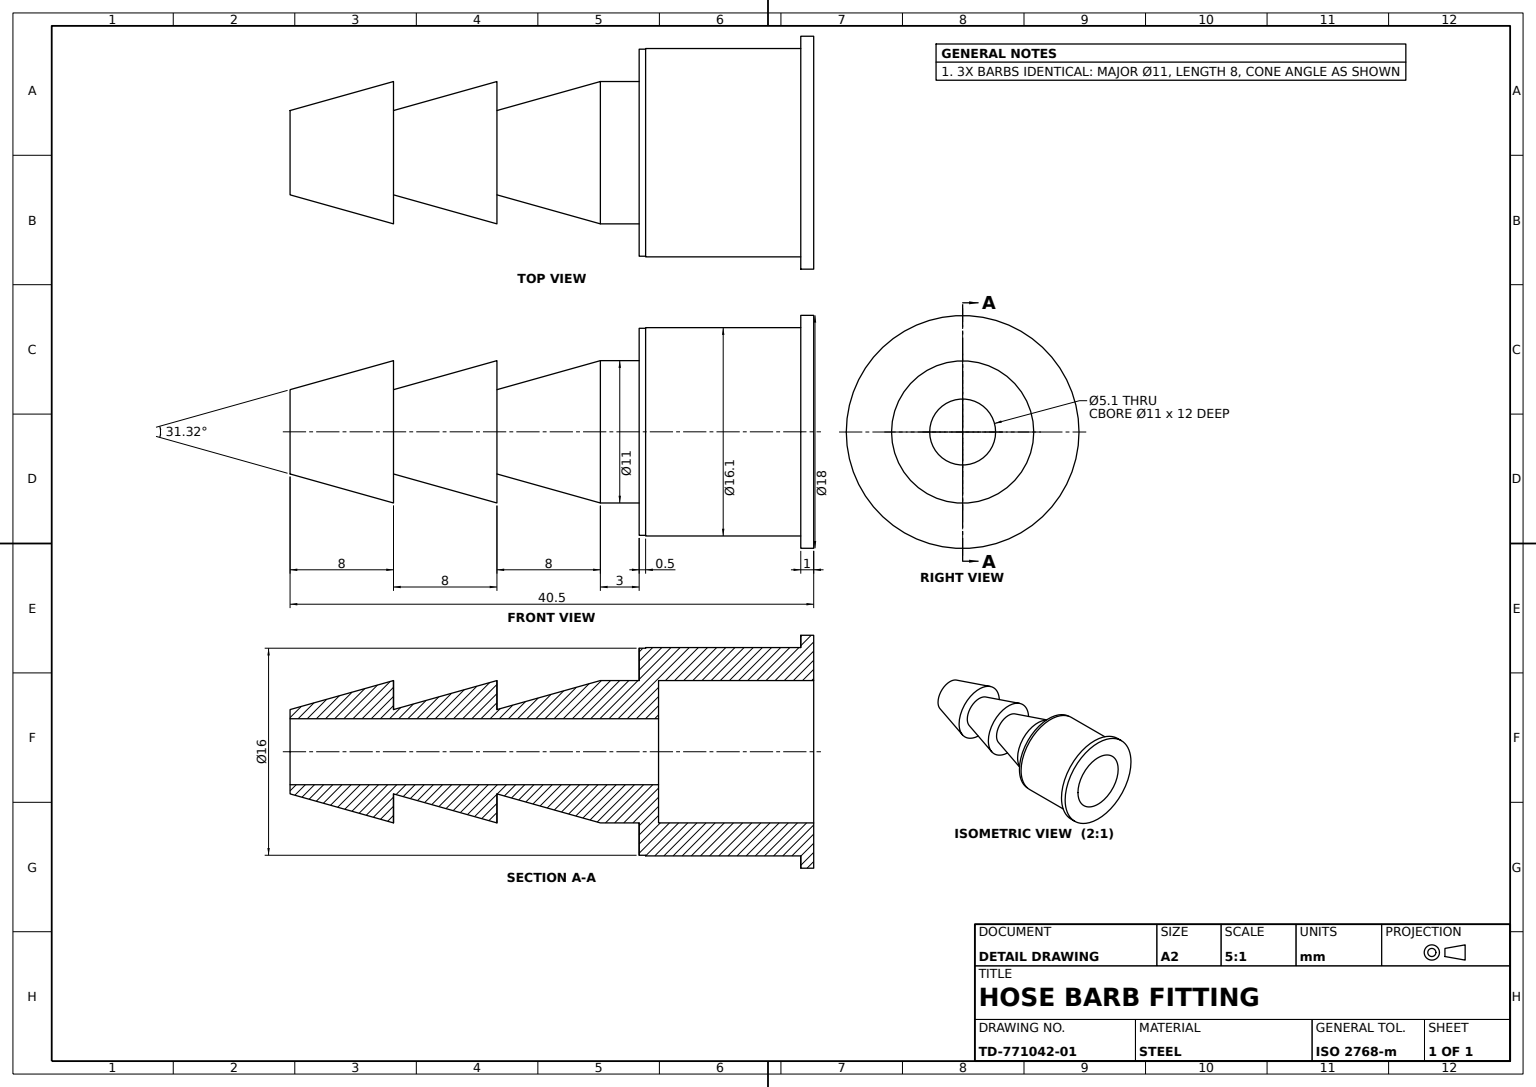
from build123d import *

# Parameters (mm, degrees)
FLANGE_SKETCH_R        = 9
FLANGE_DEPTH           = 1
BODY_SKETCH_R          = 8.05
BODY_DEPTH             = 12
SHOULDER_STEP_SKETCH_R = 8
SHOULDER_STEP_DEPTH    = 0.5
NECK_SKETCH_R          = 5.5
NECK_DEPTH             = 3
BARB_1_SKETCH_R        = 5.5
BARB_1_DEPTH           = 8
BARB_1_TAPER           = 15.66
BARB_2_SKETCH_R        = 5.5
BARB_2_DEPTH           = 8
BARB_2_TAPER           = 15.66
BARB_3_SKETCH_R        = 5.5
BARB_3_TIP_DEPTH       = 8
BARB_3_TIP_TAPER       = 15.66
INLET_BORE_SKETCH_R    = 5.5
INLET_BORE_DEPTH       = 12
THROUGH_BORE_SKETCH_R  = 2.55
THROUGH_BORE_DEPTH     = 38


with BuildPart() as part:
    # Flange Sketch → Flange (new body)
    with BuildSketch(Plane.XY):
        Circle(FLANGE_SKETCH_R)
    extrude(amount=FLANGE_DEPTH)

    # Body Sketch → Body (add)
    with BuildSketch(Plane.XY.offset(1)):
        Circle(BODY_SKETCH_R)
    extrude(amount=BODY_DEPTH)

    # Shoulder Step Sketch → Shoulder Step (add)
    with BuildSketch(Plane.XY.offset(13)):
        Circle(SHOULDER_STEP_SKETCH_R)
    extrude(amount=SHOULDER_STEP_DEPTH)

    # Neck Sketch → Neck (add)
    with BuildSketch(Plane.XY.offset(13.5)):
        Circle(NECK_SKETCH_R)
    extrude(amount=NECK_DEPTH)

    # Barb 1 Sketch → Barb 1 (add)
    with BuildSketch(Plane.XY.offset(16.5)):
        Circle(BARB_1_SKETCH_R)
    extrude(amount=BARB_1_DEPTH, taper=BARB_1_TAPER)

    # Barb 2 Sketch → Barb 2 (add)
    with BuildSketch(Plane.XY.offset(24.5)):
        Circle(BARB_2_SKETCH_R)
    extrude(amount=BARB_2_DEPTH, taper=BARB_2_TAPER)

    # Barb 3 Sketch → Barb 3 Tip (add)
    with BuildSketch(Plane.XY.offset(32.5)):
        Circle(BARB_3_SKETCH_R)
    extrude(amount=BARB_3_TIP_DEPTH, taper=BARB_3_TIP_TAPER)

    # Inlet Bore Sketch → Inlet Bore (cut)
    with BuildSketch(Plane(origin=(0, 0, 0), x_dir=(-1, 0, 0), z_dir=(0, 0, -1))):
        with Locations(Location((0, 0, 0), (0, 0, 180))):
            Circle(INLET_BORE_SKETCH_R)
    extrude(amount=-INLET_BORE_DEPTH, mode=Mode.SUBTRACT)

    # Through Bore Sketch → Through Bore (cut)
    with BuildSketch(Plane(origin=(0, 0, 12), x_dir=(-1, 0, 0), z_dir=(0, 0, -1))):
        Circle(THROUGH_BORE_SKETCH_R)
    extrude(amount=-THROUGH_BORE_DEPTH, mode=Mode.SUBTRACT)


solid = part.part
